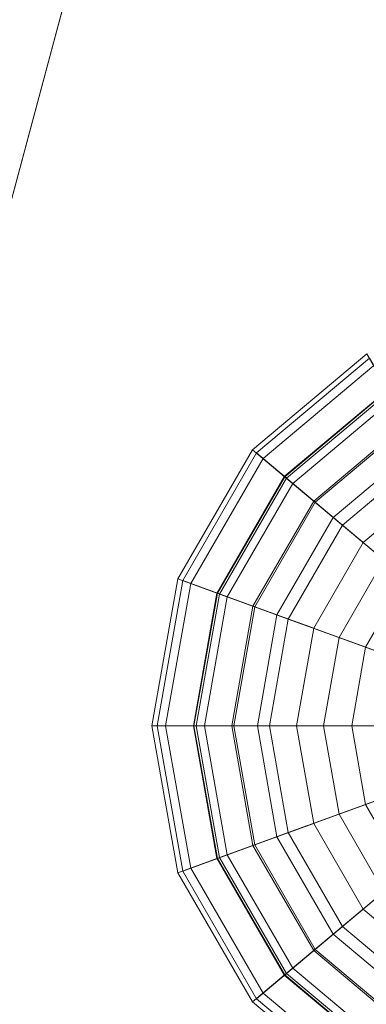
# Model space of a CAD drawing. Units: inches. Extents: x 375 to 1122, y 27 to 1069.
# Tile 21 of 155: x 717.492 to 718.584, y 272.362 to 275.466. Entities that reach past the tile are written whole.
import ezdxf

# ---------------------------------------------------------------- set-up
doc = ezdxf.new("R2010")
doc.units = ezdxf.units.IN
doc.layers.add('Furniture', color=30, linetype='Continuous', lineweight=18)

# ---------------------------------------------------------------- blocks, each defined once
blk = doc.blocks.new('A$C403C54AD')
for points in [[(1.797233, 0.840953, -0.031825), (1.826559, 0.857884, -0.028747), (1.826559, 0.857884, -0.028747), (1.804793, 0.831944, -0.031825)], [(1.804793, 0.831944, -0.031825), (1.826559, 0.857884, -0.028747), (1.826559, 0.857884, -0.028747), (1.814977, 0.826064, -0.031825)], [(1.814977, 0.826064, -0.031825), (1.826559, 0.857884, -0.028747), (1.826559, 0.857884, -0.028747), (1.826559, 0.824022, -0.031825)], [(1.848325, 0.831944, -0.031825), (1.826559, 0.857884, -0.028747), (1.826559, 0.857884, -0.028747), (1.855884, 0.840953, -0.031825)], [(1.83814, 0.826064, -0.031825), (1.826559, 0.857884, -0.028747), (1.826559, 0.857884, -0.028747), (1.848325, 0.831944, -0.031825)], [(1.826559, 0.824022, -0.031825), (1.826559, 0.857884, -0.028747), (1.826559, 0.857884, -0.028747), (1.83814, 0.826064, -0.031825)], [(1.814249, 0.850777, -0.02532), (1.800062, 0.842586, -0.028594), (1.806892, 0.834446, -0.028594), (1.817422, 0.846995, -0.02532)], [(1.820835, 0.851063, 0.057003), (1.814907, 0.843998, 0.063639), (1.820359, 0.84085, 0.063639), (1.823514, 0.849517, 0.057003)], [(1.829604, 0.849517, 0.057003), (1.832759, 0.84085, 0.063639), (1.838211, 0.843998, 0.063639), (1.832282, 0.851063, 0.057003)], [(1.835696, 0.846995, -0.02532), (1.846226, 0.834446, -0.028594), (1.853056, 0.842586, -0.028594), (1.838869, 0.850777, -0.02532)], [(1.813473, 0.842289, 0.061451), (1.820055, 0.850133, 0.054084), (1.823098, 0.848375, 0.054084), (1.819596, 0.838754, 0.061451)], [(1.833522, 0.838754, 0.061451), (1.83002, 0.848375, 0.054084), (1.833063, 0.850133, 0.054084), (1.839644, 0.842289, 0.061451)], [(1.823514, 0.849517, 0.057003), (1.820359, 0.84085, 0.063639), (1.826559, 0.839757, 0.063639), (1.826559, 0.84898, 0.057003)], [(1.826559, 0.84898, 0.057003), (1.826559, 0.839757, 0.063639), (1.832759, 0.84085, 0.063639), (1.829604, 0.849517, 0.057003)], [(1.81086, 0.84882, 0.063639), (1.805243, 0.845577, 0.073031), (1.810738, 0.839029, 0.073031), (1.814907, 0.843998, 0.063639)], [(1.819596, 0.838754, 0.061451), (1.823098, 0.848375, 0.054084), (1.826559, 0.847765, 0.054084), (1.826559, 0.837526, 0.061451)], [(1.826559, 0.837526, 0.061451), (1.826559, 0.847765, 0.054084), (1.83002, 0.848375, 0.054084), (1.833522, 0.838754, 0.061451)], [(1.838211, 0.843998, 0.063639), (1.84238, 0.839029, 0.073031), (1.847874, 0.845577, 0.073031), (1.842258, 0.84882, 0.063639)], [(1.802809, 0.844172, 0.071684), (1.808929, 0.847705, 0.061451), (1.813473, 0.842289, 0.061451), (1.808931, 0.836876, 0.071684)], [(1.844187, 0.836876, 0.071684), (1.839644, 0.842289, 0.061451), (1.844189, 0.847705, 0.061451), (1.850309, 0.844172, 0.071684)], [(1.817422, 0.846995, -0.02532), (1.806892, 0.834446, -0.028594), (1.816094, 0.829133, -0.028594), (1.821697, 0.844527, -0.02532)], [(1.83142, 0.844527, -0.02532), (1.837023, 0.829133, -0.028594), (1.846226, 0.834446, -0.028594), (1.835696, 0.846995, -0.02532)], [(1.802683, 0.844099, 0.130354), (1.80709, 0.846643, 0.140564), (1.812108, 0.840662, 0.140564), (1.808838, 0.836765, 0.130354)], [(1.80709, 0.846643, 0.140564), (1.804424, 0.845104, 0.140564), (1.81013, 0.838304, 0.140564), (1.812108, 0.840662, 0.140564)], [(1.84101, 0.840662, 0.140564), (1.842988, 0.838304, 0.140564), (1.848694, 0.845104, 0.140564), (1.846028, 0.846643, 0.140564)], [(1.84428, 0.836765, 0.130354), (1.84101, 0.840662, 0.140564), (1.846028, 0.846643, 0.140564), (1.850434, 0.844099, 0.130354)], [(1.805243, 0.845577, 0.073031), (1.80082, 0.843024, 0.090178), (1.807455, 0.835117, 0.090178), (1.810738, 0.839029, 0.073031)], [(1.84238, 0.839029, 0.073031), (1.845663, 0.835117, 0.090178), (1.852298, 0.843024, 0.090178), (1.847874, 0.845577, 0.073031)], [(1.804424, 0.845104, 0.140564), (1.800097, 0.842606, 0.131159), (1.806918, 0.834477, 0.131159), (1.81013, 0.838304, 0.140564)], [(1.821697, 0.844527, -0.02532), (1.816094, 0.829133, -0.028594), (1.826559, 0.827288, -0.028594), (1.826559, 0.84367, -0.02532)], [(1.826559, 0.84367, -0.02532), (1.826559, 0.827288, -0.028594), (1.837023, 0.829133, -0.028594), (1.83142, 0.844527, -0.02532)], [(1.842988, 0.838304, 0.140564), (1.8462, 0.834477, 0.131159), (1.853021, 0.842606, 0.131159), (1.848694, 0.845104, 0.140564)], [(1.798163, 0.84149, 0.089693), (1.802809, 0.844172, 0.071684), (1.808931, 0.836876, 0.071684), (1.805483, 0.832767, 0.089693)], [(1.80025, 0.842695, 0.117718), (1.802683, 0.844099, 0.130354), (1.808838, 0.836765, 0.130354), (1.807032, 0.834612, 0.117718)], [(1.814907, 0.843998, 0.063639), (1.810738, 0.839029, 0.073031), (1.818141, 0.834755, 0.073031), (1.820359, 0.84085, 0.063639)], [(1.832759, 0.84085, 0.063639), (1.834977, 0.834755, 0.073031), (1.84238, 0.839029, 0.073031), (1.838211, 0.843998, 0.063639)], [(1.847635, 0.832767, 0.089693), (1.844187, 0.836876, 0.071684), (1.850309, 0.844172, 0.071684), (1.854954, 0.84149, 0.089693)], [(1.846086, 0.834612, 0.117718), (1.84428, 0.836765, 0.130354), (1.850434, 0.844099, 0.130354), (1.852868, 0.842695, 0.117718)], [(1.80082, 0.843024, 0.090178), (1.80025, 0.842695, 0.117718), (1.807032, 0.834612, 0.117718), (1.807455, 0.835117, 0.090178)], [(1.845663, 0.835117, 0.090178), (1.846086, 0.834612, 0.117718), (1.852868, 0.842695, 0.117718), (1.852298, 0.843024, 0.090178)], [(1.800062, 0.842586, -0.028594), (1.797233, 0.840953, -0.031825), (1.804793, 0.831944, -0.031825), (1.806892, 0.834446, -0.028594)], [(1.800097, 0.842606, 0.131159), (1.797579, 0.841152, 0.117935), (1.805049, 0.83225, 0.117935), (1.806918, 0.834477, 0.131159)], [(1.808931, 0.836876, 0.071684), (1.813473, 0.842289, 0.061451), (1.819596, 0.838754, 0.061451), (1.817179, 0.832114, 0.071684)], [(1.835938, 0.832114, 0.071684), (1.833522, 0.838754, 0.061451), (1.839644, 0.842289, 0.061451), (1.844187, 0.836876, 0.071684)], [(1.8462, 0.834477, 0.131159), (1.848069, 0.83225, 0.117935), (1.855539, 0.841152, 0.117935), (1.853021, 0.842606, 0.131159)], [(1.846226, 0.834446, -0.028594), (1.848325, 0.831944, -0.031825), (1.855884, 0.840953, -0.031825), (1.853056, 0.842586, -0.028594)], [(1.797579, 0.841152, 0.117935), (1.798163, 0.84149, 0.089693), (1.805483, 0.832767, 0.089693), (1.805049, 0.83225, 0.117935)], [(1.848069, 0.83225, 0.117935), (1.847635, 0.832767, 0.089693), (1.854954, 0.84149, 0.089693), (1.855539, 0.841152, 0.117935)], [(1.808838, 0.836765, 0.130354), (1.812108, 0.840662, 0.140564), (1.81887, 0.836759, 0.140564), (1.81713, 0.831977, 0.130354)], [(1.812108, 0.840662, 0.140564), (1.81013, 0.838304, 0.140564), (1.817817, 0.833866, 0.140564), (1.81887, 0.836759, 0.140564)], [(1.820359, 0.84085, 0.063639), (1.818141, 0.834755, 0.073031), (1.826559, 0.833271, 0.073031), (1.826559, 0.839757, 0.063639)], [(1.826559, 0.839757, 0.063639), (1.826559, 0.833271, 0.073031), (1.834977, 0.834755, 0.073031), (1.832759, 0.84085, 0.063639)], [(1.834248, 0.836759, 0.140564), (1.835301, 0.833866, 0.140564), (1.842988, 0.838304, 0.140564), (1.84101, 0.840662, 0.140564)], [(1.835988, 0.831977, 0.130354), (1.834248, 0.836759, 0.140564), (1.84101, 0.840662, 0.140564), (1.84428, 0.836765, 0.130354)], [(1.810738, 0.839029, 0.073031), (1.807455, 0.835117, 0.090178), (1.816394, 0.829956, 0.090178), (1.818141, 0.834755, 0.073031)], [(1.834977, 0.834755, 0.073031), (1.836724, 0.829956, 0.090178), (1.845663, 0.835117, 0.090178), (1.84238, 0.839029, 0.073031)], [(1.81013, 0.838304, 0.140564), (1.806918, 0.834477, 0.131159), (1.816108, 0.829171, 0.131159), (1.817817, 0.833866, 0.140564)], [(1.817179, 0.832114, 0.071684), (1.819596, 0.838754, 0.061451), (1.826559, 0.837526, 0.061451), (1.826559, 0.83046, 0.071684)], [(1.826559, 0.83046, 0.071684), (1.826559, 0.837526, 0.061451), (1.833522, 0.838754, 0.061451), (1.835938, 0.832114, 0.071684)], [(1.835301, 0.833866, 0.140564), (1.83701, 0.829171, 0.131159), (1.8462, 0.834477, 0.131159), (1.842988, 0.838304, 0.140564)], [(1.805483, 0.832767, 0.089693), (1.808931, 0.836876, 0.071684), (1.817179, 0.832114, 0.071684), (1.815345, 0.827073, 0.089693)], [(1.807032, 0.834612, 0.117718), (1.808838, 0.836765, 0.130354), (1.81713, 0.831977, 0.130354), (1.816169, 0.829337, 0.117718)], [(1.81713, 0.831977, 0.130354), (1.81887, 0.836759, 0.140564), (1.826559, 0.835403, 0.140564), (1.826559, 0.830315, 0.130354)], [(1.81887, 0.836759, 0.140564), (1.817817, 0.833866, 0.140564), (1.826559, 0.832324, 0.140564), (1.826559, 0.835403, 0.140564)], [(1.826559, 0.835403, 0.140564), (1.826559, 0.832324, 0.140564), (1.835301, 0.833866, 0.140564), (1.834248, 0.836759, 0.140564)], [(1.826559, 0.830315, 0.130354), (1.826559, 0.835403, 0.140564), (1.834248, 0.836759, 0.140564), (1.835988, 0.831977, 0.130354)], [(1.837773, 0.827073, 0.089693), (1.835938, 0.832114, 0.071684), (1.844187, 0.836876, 0.071684), (1.847635, 0.832767, 0.089693)], [(1.836949, 0.829337, 0.117718), (1.835988, 0.831977, 0.130354), (1.84428, 0.836765, 0.130354), (1.846086, 0.834612, 0.117718)], [(1.806892, 0.834446, -0.028594), (1.804793, 0.831944, -0.031825), (1.814977, 0.826064, -0.031825), (1.816094, 0.829133, -0.028594)], [(1.806918, 0.834477, 0.131159), (1.805049, 0.83225, 0.117935), (1.815114, 0.826439, 0.117935), (1.816108, 0.829171, 0.131159)], [(1.807455, 0.835117, 0.090178), (1.807032, 0.834612, 0.117718), (1.816169, 0.829337, 0.117718), (1.816394, 0.829956, 0.090178)], [(1.818141, 0.834755, 0.073031), (1.816394, 0.829956, 0.090178), (1.826559, 0.828163, 0.090178), (1.826559, 0.833271, 0.073031)], [(1.826559, 0.833271, 0.073031), (1.826559, 0.828163, 0.090178), (1.836724, 0.829956, 0.090178), (1.834977, 0.834755, 0.073031)], [(1.836724, 0.829956, 0.090178), (1.836949, 0.829337, 0.117718), (1.846086, 0.834612, 0.117718), (1.845663, 0.835117, 0.090178)], [(1.83701, 0.829171, 0.131159), (1.838004, 0.826439, 0.117935), (1.848069, 0.83225, 0.117935), (1.8462, 0.834477, 0.131159)], [(1.837023, 0.829133, -0.028594), (1.83814, 0.826064, -0.031825), (1.848325, 0.831944, -0.031825), (1.846226, 0.834446, -0.028594)], [(1.817817, 0.833866, 0.140564), (1.816108, 0.829171, 0.131159), (1.826559, 0.827328, 0.131159), (1.826559, 0.832324, 0.140564)], [(1.826559, 0.832324, 0.140564), (1.826559, 0.827328, 0.131159), (1.83701, 0.829171, 0.131159), (1.835301, 0.833866, 0.140564)], [(1.805049, 0.83225, 0.117935), (1.805483, 0.832767, 0.089693), (1.815345, 0.827073, 0.089693), (1.815114, 0.826439, 0.117935)], [(1.815345, 0.827073, 0.089693), (1.817179, 0.832114, 0.071684), (1.826559, 0.83046, 0.071684), (1.826559, 0.825096, 0.089693)], [(1.826559, 0.825096, 0.089693), (1.826559, 0.83046, 0.071684), (1.835938, 0.832114, 0.071684), (1.837773, 0.827073, 0.089693)], [(1.838004, 0.826439, 0.117935), (1.837773, 0.827073, 0.089693), (1.847635, 0.832767, 0.089693), (1.848069, 0.83225, 0.117935)], [(1.816169, 0.829337, 0.117718), (1.81713, 0.831977, 0.130354), (1.826559, 0.830315, 0.130354), (1.826559, 0.827505, 0.117718)], [(1.826559, 0.827505, 0.117718), (1.826559, 0.830315, 0.130354), (1.835988, 0.831977, 0.130354), (1.836949, 0.829337, 0.117718)], [(1.816394, 0.829956, 0.090178), (1.816169, 0.829337, 0.117718), (1.826559, 0.827505, 0.117718), (1.826559, 0.828163, 0.090178)], [(1.826559, 0.828163, 0.090178), (1.826559, 0.827505, 0.117718), (1.836949, 0.829337, 0.117718), (1.836724, 0.829956, 0.090178)], [(1.816094, 0.829133, -0.028594), (1.814977, 0.826064, -0.031825), (1.826559, 0.824022, -0.031825), (1.826559, 0.827288, -0.028594)], [(1.816108, 0.829171, 0.131159), (1.815114, 0.826439, 0.117935), (1.826559, 0.824421, 0.117935), (1.826559, 0.827328, 0.131159)], [(1.826559, 0.827328, 0.131159), (1.826559, 0.824421, 0.117935), (1.838004, 0.826439, 0.117935), (1.83701, 0.829171, 0.131159)], [(1.826559, 0.827288, -0.028594), (1.826559, 0.824022, -0.031825), (1.83814, 0.826064, -0.031825), (1.837023, 0.829133, -0.028594)], [(1.815114, 0.826439, 0.117935), (1.815345, 0.827073, 0.089693), (1.826559, 0.825096, 0.089693), (1.826559, 0.824421, 0.117935)], [(1.826559, 0.824421, 0.117935), (1.826559, 0.825096, 0.089693), (1.837773, 0.827073, 0.089693), (1.838004, 0.826439, 0.117935)]]:
    blk.add_3dface(points)
at = {"linetype": 'ByBlock', "invisible_edges": 5}
for points in [[(1.795775, 0.81008, -0.008737), (1.78654, 0.794084, -0.008737), (1.726512, 0.810169, -0.008737), (1.726512, 0.828639, -0.008737)], [(1.778844, 0.780755, -0.02259), (1.795775, 0.81008, -0.013355), (1.726512, 0.828639, -0.013355), (1.726512, 0.794777, -0.02259)]]:
    blk.add_3dface(points, dxfattribs=at)
at = {"linetype": 'ByBlock'}
blk.add_3dface([(1.795775, 0.81008, -0.013355), (1.795775, 0.81008, -0.008737), (1.726512, 0.828639, -0.008737), (1.726512, 0.828639, -0.013355)], dxfattribs=at)

msp = doc.modelspace()

# ---------------------------------------------------------------- block references
at = {"layer": 'Furniture', "xscale": 39.9918517141215, "yscale": 39.9918517141215, "zscale": 39.9918517141215, "rotation": 270}
msp.add_blockref('A$C403C54AD', (684.9549, 346.2875, 0.024), dxfattribs=at)

doc.saveas('drawing.dxf')
